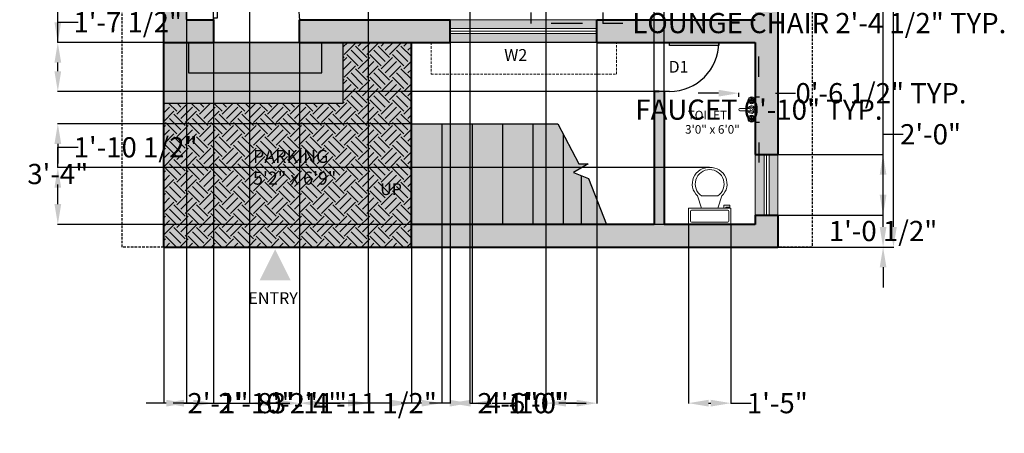
# Model space of a CAD drawing. Units: inches. Extents: x 277 to 728, y 649 to 1132.
# Tile 1 of 4: x 285 to 674, y 649 to 813. Entities that reach past the tile are written whole.
import ezdxf

# ---------------------------------------------------------------- set-up
doc = ezdxf.new("R2010")
doc.units = ezdxf.units.IN
doc.header["$MEASUREMENT"] = 0
doc.linetypes.add('DASHEDX2', pattern=[1.5, 1, -0.5])
for name, color, linetype, lineweight in [('A-ANNO-DIMS', 2, 'Continuous', 18), ('A-ANNO-SYMB', 7, 'Continuous', 18), ('A-ANNO-TEXT', 7, 'Continuous', 18), ('A-AREA-IDEN', 7, 'Continuous', 25), ('A-DOOR', 3, 'Continuous', 25), ('A-FLOR-FIXT', 8, 'Continuous', 18), ('A-FLOR-STRS', 7, 'Continuous', 25), ('A-FLOR-STRS-PATT', 252, 'Continuous', 9), ('A-GLAZ', 4, 'Continuous', 18), ('A-GLAZ-OVHD', 8, 'DASHEDX2', 13), ('A-WALL', 7, 'Continuous', 40), ('A-WALL-PATT', 8, 'Continuous', 13), ('C-PROP', 7, 'DASHEDX2', 25)]:
    doc.layers.add(name, color=color, linetype=linetype, lineweight=lineweight)
for name, color, linetype, lineweight, true_color in [('A-FLOR-FNSH-PATT', 144, 'Continuous', 9, 0x1e788f), ('A-FLOR-PATT', 39, 'Continuous', 9, 0x603913), ('A-GLAZ-PATT', 144, 'Continuous', 13, 0x1e788f)]:
    doc.layers.add(name, color=color, linetype=linetype, lineweight=lineweight, true_color=true_color)
doc.styles.get("Standard").update_dxf_attribs({"font": 'arial.ttf'})
doc.dimstyles.get("Standard").update_dxf_attribs({"dimtxt": 8, "dimasz": 8, "dimexe": 0.18, "dimexo": 0.0625, "dimgap": 0.09, "dimtad": 0, "dimtih": 1, "dimtoh": 1, "dimdec": 0, "dimzin": 0, "dimdsep": 46, "dimlunit": 3, "dimtxsty": 'Standard', "dimcen": 0.09, "dimadec": 0, "dimazin": 0, "dimtfac": 1, "dimtdec": 0, "dimtofl": 0, "dimtmove": 0, "dimatfit": 3, "dimfxl": 1, "dimtolj": 1, "dimtzin": 0, "dimarcsym": 0})

# ---------------------------------------------------------------- blocks, each defined once
blk = doc.blocks.new('*U4')
for p, q in [((0, 0), (0, -6)), ((40, 0), (40, -6))]:
    blk.add_line(p, q)
blk.add_lwpolyline([(0, 0), (0, 40), (1.75, 40), (1.75, 0)], close=True)
blk.add_arc((0, 0), 40, 0, 90)
blk = doc.blocks.new('*U5')
for p, q in [((0, 0), (0, -6)), ((28, 0), (28, -6))]:
    blk.add_line(p, q)
blk.add_lwpolyline([(0, 0), (0, 28), (1.75, 28), (1.75, 0)], close=True)
blk.add_arc((0, 0), 28, 0, 90)
blk = doc.blocks.new('*U16')
for p, q in [((9.5, -6), (9.5, -2)), ((-10, -8.5), (-8, -8.5)), ((-10, -9.5), (-10, -8.5)), ((-7, -9.5), (-10, -9.5)), ((-8, -8.5), (-8, -8)), ((-7, -8), (-7, -9.5)), ((-4, -8), (-6, -14)), ((4, -8), (6, -14)), ((4, -14), (-4, -14))]:
    blk.add_line(p, q)
blk.add_lwpolyline([(10.5, -8), (10.5, 0), (-10.5, 0), (-10.5, -8)], close=True)
for points in [[(-9.5, -2), (-9.5, -6)], [(8.5, -1), (-8.5, -1)], [(-8.5, -7), (8.5, -7)]]:
    blk.add_lwpolyline(points)
for centre, radius, start, end in [((-8.625, -1.875), 0.8839, 81.8699, 188.1301), ((8.625, -1.875), 0.8839, 351.8699, 98.1301), ((-8.625, -6.125), 0.8839, 171.869898, 278.1301), ((8.625, -6.125), 0.8839, 261.8699, 8.1301), ((-0.4772, -19.9188), 8.0953, 133.01722, 273.38), ((0.0374, -19.8731), 7.127, 124.50543, 269.7), ((-0.0373, -19.8731), 7.127, 270.3, 55.4946), ((0.4773, -19.9188), 8.0953, 266.62, 46.9828)]:
    blk.add_arc(centre, radius, start, end)
blk = doc.blocks.new('Faucet - Bathroom top')
for p, q in [((-4.107, 0.125), (-4.375, 0.125)), ((-3.75, 0.4788), (-3.75, 0.75)), ((-3.5, 0.482), (-3.5, 0.75)), ((-3.1461, 0.125), (-2.875, 0.125)), ((3.143, 0.125), (2.875, 0.125)), ((3.5, 0.4788), (3.5, 0.75)), ((3.75, 0.482), (3.75, 0.75)), ((4.1039, 0.125), (4.375, 0.125)), ((-4.1039, -0.125), (-4.375, -0.125)), ((-3.75, -0.4821), (-3.75, -0.75)), ((-3.5, -0.4789), (-3.5, -0.75)), ((-3.143, -0.125), (-2.875, -0.125)), ((-0.5, -0.8639), (-0.5, -4.5)), ((0.5, -4.5), (0.5, -0.8631)), ((3.1461, -0.125), (2.875, -0.125)), ((3.5, -0.4821), (3.5, -0.75)), ((3.75, -0.4789), (3.75, -0.75)), ((4.107, -0.125), (4.375, -0.125))]:
    blk.add_line(p, q)
for centre, radius in [((-3.625, 0), 1.375), ((-4.625, 0), 0.2795), ((-3.625, 0), 0.5), ((-3.625, 1), 0.2795), ((-2.625, 0), 0.2795), ((0, 0), 0.5), ((3.625, 0), 1.375), ((2.625, 0), 0.2795), ((3.625, 0), 0.5), ((3.625, 1), 0.2795), ((4.625, 0), 0.2795), ((-3.625, -1), 0.2795), ((3.625, -1), 0.2795)]:
    blk.add_circle(centre, radius)
for centre, radius, start, end in [((-3.625, 0), 1, 105.2407, 164.2093), ((-3.625, 0), 1, 16.44125, 74.07887), ((0, 0), 1.5, 289.6514, 250.3603), ((0, 0), 1, 300.3431, 239.7554), ((3.625, 0), 1, 106.12, 164.0884), ((3.625, 0), 1, 16.23422, 73.90469), ((-3.625, 0), 1, 196.2342, 253.9047), ((-3.625, 0), 1, 286.12, 344.0884), ((3.625, 0), 1, 196.4413, 254.0789), ((3.625, 0), 1, 285.2407, 344.2093), ((0, -4.5), 0.5, 180, 0)]:
    blk.add_arc(centre, radius, start, end)
blk = doc.blocks.new('Moment Connection - Imperial')
at = {"color": 0}
blk.add_solid([(0, 0.125), (0.125, 0.0625), (0, 0)], dxfattribs=at)
blk = doc.blocks.new('*D21')
at = {"layer": 'A-ANNO-DIMS', "color": 0, "lineweight": -2, "transparency": 16777216}
for p, q in [((598.28, 1083.05), (630.62, 1083.05)), ((630.44, 1075.05), (630.44, 907.23)), ((630.44, 731.05), (630.44, 898.87)), ((598.28, 723.05), (630.62, 723.05))]:
    blk.add_line(p, q, dxfattribs=at)
at = {"layer": 'A-ANNO-DIMS', "color": 0, "transparency": 16777216}
for points in [[(629.11, 1075.05), (631.77, 1075.05), (630.44, 1083.05)], [(629.11, 731.05), (631.77, 731.05), (630.44, 723.05)]]:
    blk.add_solid(points, dxfattribs=at)
at = {"layer": 'Defpoints', "color": 0, "transparency": 16777216}
for p in [(598.22, 1083.05), (598.22, 723.05), (630.44, 723.05)]:
    blk.add_point(p, dxfattribs=at)
at = {"layer": 'A-ANNO-DIMS', "color": 0, "transparency": 16777216, "insert": (630.44, 903.05), "char_height": 8, "attachment_point": 5}
blk.add_mtext("\\A1;30'", dxfattribs=at)
blk = doc.blocks.new('*D27')
at = {"layer": 'A-ANNO-DIMS', "color": 0, "lineweight": -2, "transparency": 16777216}
for p, q in [((577.22, 790.46), (577.22, 798.46)), ((575.78, 782.46), (577.4, 782.46)), ((575.78, 772.46), (577.4, 772.46)), ((577.22, 764.46), (577.22, 756.46))]:
    blk.add_line(p, q, dxfattribs=at)
at = {"layer": 'A-ANNO-DIMS', "color": 0, "transparency": 16777216}
for points in [[(575.89, 790.46), (578.55, 790.46), (577.22, 782.46)], [(575.89, 764.46), (578.55, 764.46), (577.22, 772.46)]]:
    blk.add_solid(points, dxfattribs=at)
at = {"layer": 'Defpoints', "color": 0, "transparency": 16777216}
for p in [(575.72, 782.46), (575.72, 772.46), (577.22, 772.46)]:
    blk.add_point(p, dxfattribs=at)
at = {"layer": 'A-ANNO-DIMS', "color": 0, "transparency": 16777216, "insert": (577.22, 777.46), "char_height": 8, "attachment_point": 5}
blk.add_mtext('\\A1;FAUCET 0\'-10" TYP.', dxfattribs=at)
blk = doc.blocks.new('*D28')
at = {"layer": 'A-ANNO-DIMS', "color": 0, "lineweight": -2, "transparency": 16777216}
for p, q in [((561.22, 783.96), (553.22, 783.96)), ((569.22, 782.52), (569.22, 784.14)), ((575.72, 782.52), (575.72, 784.14)), ((583.72, 783.96), (591.72, 783.96))]:
    blk.add_line(p, q, dxfattribs=at)
at = {"layer": 'A-ANNO-DIMS', "color": 0, "transparency": 16777216}
for points in [[(561.22, 785.29), (561.22, 782.62), (569.22, 783.96)], [(583.72, 785.29), (583.72, 782.62), (575.72, 783.96)]]:
    blk.add_solid(points, dxfattribs=at)
at = {"layer": 'Defpoints', "color": 0, "transparency": 16777216}
for p in [(575.72, 783.96), (569.22, 782.46), (575.72, 782.46)]:
    blk.add_point(p, dxfattribs=at)
at = {"layer": 'A-ANNO-DIMS', "color": 0, "transparency": 16777216, "insert": (625.51, 783.96), "char_height": 8, "attachment_point": 5}
blk.add_mtext('\\A1;0\'-6 1/2" TYP.', dxfattribs=at)
blk = doc.blocks.new('*D29')
at = {"layer": 'A-ANNO-DIMS', "color": 0, "lineweight": -2, "transparency": 16777216}
for p, q in [((486.97, 815.91), (486.97, 811.53)), ((515.41, 815.91), (515.41, 811.53)), ((494.97, 811.71), (507.41, 811.71)), ((515.41, 811.71), (523.41, 811.71))]:
    blk.add_line(p, q, dxfattribs=at)
at = {"layer": 'A-ANNO-DIMS', "color": 0, "transparency": 16777216}
for points in [[(494.97, 813.04), (494.97, 810.37), (486.97, 811.71)], [(507.41, 813.04), (507.41, 810.37), (515.41, 811.71)]]:
    blk.add_solid(points, dxfattribs=at)
at = {"layer": 'Defpoints', "color": 0, "transparency": 16777216}
for p in [(486.97, 815.97), (515.41, 815.97), (515.41, 811.71)]:
    blk.add_point(p, dxfattribs=at)
at = {"layer": 'A-ANNO-DIMS', "color": 0, "transparency": 16777216, "insert": (601.11, 811.71), "char_height": 8, "attachment_point": 5}
blk.add_mtext('\\A1;LOUNGE CHAIR 2\'-4 1/2" TYP.', dxfattribs=at)
blk = doc.blocks.new('*D48')
at = {"layer": 'A-ANNO-DIMS', "color": 0, "lineweight": -2, "transparency": 16777216}
for p, q in [((584.78, 1071.05), (626.51, 1071.05)), ((626.33, 1063.05), (626.33, 901.23)), ((626.33, 731.05), (626.33, 892.88)), ((584.78, 723.05), (626.51, 723.05))]:
    blk.add_line(p, q, dxfattribs=at)
at = {"layer": 'A-ANNO-DIMS', "color": 0, "transparency": 16777216}
for points in [[(625, 1063.05), (627.67, 1063.05), (626.33, 1071.05)], [(625, 731.05), (627.67, 731.05), (626.33, 723.05)]]:
    blk.add_solid(points, dxfattribs=at)
at = {"layer": 'Defpoints', "color": 0, "transparency": 16777216}
for p in [(584.72, 1071.05), (626.33, 1071.05), (584.72, 723.05)]:
    blk.add_point(p, dxfattribs=at)
at = {"layer": 'A-ANNO-DIMS', "color": 0, "transparency": 16777216, "insert": (626.33, 897.05), "char_height": 8, "attachment_point": 5}
blk.add_mtext('\\A1;29\'-0"', dxfattribs=at)
blk = doc.blocks.new('*D52')
at = {"layer": 'A-ANNO-DIMS', "color": 0, "lineweight": -2, "transparency": 16777216}
for p, q in [((341.66, 942.05), (299.63, 942.05)), ((299.81, 934.05), (299.81, 877.23)), ((299.81, 812.05), (299.81, 868.88)), ((341.66, 804.05), (299.63, 804.05))]:
    blk.add_line(p, q, dxfattribs=at)
at = {"layer": 'A-ANNO-DIMS', "color": 0, "transparency": 16777216}
for points in [[(298.48, 934.05), (301.15, 934.05), (299.81, 942.05)], [(298.48, 812.05), (301.15, 812.05), (299.81, 804.05)]]:
    blk.add_solid(points, dxfattribs=at)
at = {"layer": 'Defpoints', "color": 0, "transparency": 16777216}
for p in [(299.81, 942.05), (341.72, 942.05), (341.72, 804.05)]:
    blk.add_point(p, dxfattribs=at)
at = {"layer": 'A-ANNO-DIMS', "color": 0, "transparency": 16777216, "insert": (299.81, 873.05), "char_height": 8, "attachment_point": 5}
blk.add_mtext('\\A1;11\'-6"', dxfattribs=at)
blk = doc.blocks.new('*D55')
at = {"layer": 'A-ANNO-DIMS', "color": 0, "lineweight": -2, "transparency": 16777216}
for p, q in [((626.33, 759.7), (626.33, 767.7)), ((626.33, 767.7), (634.33, 767.7)), ((584.78, 759.7), (626.51, 759.7)), ((626.33, 743.74), (626.33, 751.7)), ((584.78, 735.74), (626.51, 735.74))]:
    blk.add_line(p, q, dxfattribs=at)
at = {"layer": 'A-ANNO-DIMS', "color": 0, "transparency": 16777216}
for points in [[(625, 751.7), (627.67, 751.7), (626.33, 759.7)], [(625, 743.74), (627.67, 743.74), (626.33, 735.74)]]:
    blk.add_solid(points, dxfattribs=at)
at = {"layer": 'Defpoints', "color": 0, "transparency": 16777216}
for p in [(584.72, 759.7), (626.33, 759.7), (584.72, 735.74)]:
    blk.add_point(p, dxfattribs=at)
at = {"layer": 'A-ANNO-DIMS', "color": 0, "transparency": 16777216, "insert": (645.12, 767.7), "char_height": 8, "attachment_point": 5}
blk.add_mtext('\\A1;2\'-0"', dxfattribs=at)
blk = doc.blocks.new('*D56')
at = {"layer": 'A-ANNO-DIMS', "color": 0, "lineweight": -2, "transparency": 16777216}
for p, q in [((626.33, 743.74), (626.33, 751.74)), ((584.78, 735.74), (626.51, 735.74)), ((584.78, 723.05), (626.51, 723.05)), ((626.33, 715.05), (626.33, 707.05))]:
    blk.add_line(p, q, dxfattribs=at)
at = {"layer": 'A-ANNO-DIMS', "color": 0, "transparency": 16777216}
for points in [[(625, 743.74), (627.67, 743.74), (626.33, 735.74)], [(625, 715.05), (627.67, 715.05), (626.33, 723.05)]]:
    blk.add_solid(points, dxfattribs=at)
at = {"layer": 'Defpoints', "color": 0, "transparency": 16777216}
for p in [(584.72, 735.74), (626.33, 735.74), (584.72, 723.05)]:
    blk.add_point(p, dxfattribs=at)
at = {"layer": 'A-ANNO-DIMS', "color": 0, "transparency": 16777216, "insert": (626.33, 729.4), "char_height": 8, "attachment_point": 5}
blk.add_mtext('\\A1;1\'-0 1/2"', dxfattribs=at)
blk = doc.blocks.new('*D57')
at = {"layer": 'A-ANNO-DIMS', "color": 0, "lineweight": -2, "transparency": 16777216}
for p, q in [((341.72, 722.99), (341.72, 661.09)), ((439.72, 722.99), (439.72, 661.09)), ((349.72, 661.27), (379.99, 661.27)), ((431.72, 661.27), (401.45, 661.27))]:
    blk.add_line(p, q, dxfattribs=at)
at = {"layer": 'A-ANNO-DIMS', "color": 0, "transparency": 16777216}
for points in [[(349.72, 662.6), (349.72, 659.93), (341.72, 661.27)], [(431.72, 662.6), (431.72, 659.93), (439.72, 661.27)]]:
    blk.add_solid(points, dxfattribs=at)
at = {"layer": 'Defpoints', "color": 0, "transparency": 16777216}
for p in [(341.72, 723.05), (439.72, 723.05), (439.72, 661.27)]:
    blk.add_point(p, dxfattribs=at)
at = {"layer": 'A-ANNO-DIMS', "color": 0, "transparency": 16777216, "insert": (390.72, 661.27), "char_height": 8, "attachment_point": 5}
blk.add_mtext('\\A1;8\'-2"', dxfattribs=at)
blk = doc.blocks.new('*D58')
at = {"layer": 'A-ANNO-DIMS', "color": 0, "lineweight": -2, "transparency": 16777216}
for p, q in [((342.72, 1117.04), (334.72, 1117.04)), ((350.72, 813.11), (350.72, 1117.22)), ((361.43, 813.11), (361.43, 1117.22)), ((369.43, 1117.04), (377.43, 1117.04))]:
    blk.add_line(p, q, dxfattribs=at)
at = {"layer": 'A-ANNO-DIMS', "color": 0, "transparency": 16777216}
for points in [[(342.72, 1118.37), (342.72, 1115.71), (350.72, 1117.04)], [(369.43, 1118.37), (369.43, 1115.71), (361.43, 1117.04)]]:
    blk.add_solid(points, dxfattribs=at)
at = {"layer": 'Defpoints', "color": 0, "transparency": 16777216}
for p in [(361.43, 1117.04), (350.72, 813.05), (361.43, 813.05)]:
    blk.add_point(p, dxfattribs=at)
at = {"layer": 'A-ANNO-DIMS', "color": 0, "transparency": 16777216, "insert": (400.59, 1117.04), "char_height": 8, "attachment_point": 5}
blk.add_mtext('\\A1;0\'-10 1/2"', dxfattribs=at)
blk = doc.blocks.new('*D59')
at = {"layer": 'A-ANNO-DIMS', "color": 0, "lineweight": -2, "transparency": 16777216}
for p, q in [((361.43, 803.99), (361.43, 661.09)), ((395.5, 803.99), (395.5, 661.09)), ((353.43, 661.27), (345.43, 661.27)), ((403.5, 661.27), (411.5, 661.27))]:
    blk.add_line(p, q, dxfattribs=at)
at = {"layer": 'A-ANNO-DIMS', "color": 0, "transparency": 16777216}
for points in [[(353.43, 662.6), (353.43, 659.93), (361.43, 661.27)], [(403.5, 662.6), (403.5, 659.93), (395.5, 661.27)]]:
    blk.add_solid(points, dxfattribs=at)
at = {"layer": 'Defpoints', "color": 0, "transparency": 16777216}
for p in [(361.43, 804.05), (395.5, 804.05), (395.5, 661.27)]:
    blk.add_point(p, dxfattribs=at)
at = {"layer": 'A-ANNO-DIMS', "color": 0, "transparency": 16777216, "insert": (378.46, 661.27), "char_height": 8, "attachment_point": 5}
blk.add_mtext('\\A1;2\'-10"', dxfattribs=at)
blk = doc.blocks.new('*D60')
at = {"layer": 'A-ANNO-DIMS', "color": 0, "lineweight": -2, "transparency": 16777216}
for p, q in [((395.5, 803.99), (395.5, 661.09)), ((455.1, 803.99), (455.1, 661.09)), ((387.5, 661.27), (379.5, 661.27)), ((463.1, 661.27), (471.1, 661.27))]:
    blk.add_line(p, q, dxfattribs=at)
at = {"layer": 'A-ANNO-DIMS', "color": 0, "transparency": 16777216}
for points in [[(387.5, 662.6), (387.5, 659.93), (395.5, 661.27)], [(463.1, 662.6), (463.1, 659.93), (455.1, 661.27)]]:
    blk.add_solid(points, dxfattribs=at)
at = {"layer": 'Defpoints', "color": 0, "transparency": 16777216}
for p in [(395.5, 804.05), (455.1, 804.05), (455.1, 661.27)]:
    blk.add_point(p, dxfattribs=at)
at = {"layer": 'A-ANNO-DIMS', "color": 0, "transparency": 16777216, "insert": (425.3, 661.27), "char_height": 8, "attachment_point": 5}
blk.add_mtext('\\A1;4\'-11 1/2"', dxfattribs=at)
blk = doc.blocks.new('*D61')
at = {"layer": 'A-ANNO-DIMS', "color": 0, "lineweight": -2, "transparency": 16777216}
for p, q in [((455.1, 803.99), (455.1, 661.09)), ((513.09, 803.99), (513.09, 661.09)), ((463.1, 661.27), (470.11, 661.27)), ((505.09, 661.27), (498.09, 661.27))]:
    blk.add_line(p, q, dxfattribs=at)
at = {"layer": 'A-ANNO-DIMS', "color": 0, "transparency": 16777216}
for points in [[(463.1, 662.6), (463.1, 659.93), (455.1, 661.27)], [(505.09, 662.6), (505.09, 659.93), (513.09, 661.27)]]:
    blk.add_solid(points, dxfattribs=at)
at = {"layer": 'Defpoints', "color": 0, "transparency": 16777216}
for p in [(455.1, 804.05), (513.09, 804.05), (513.09, 661.27)]:
    blk.add_point(p, dxfattribs=at)
at = {"layer": 'A-ANNO-DIMS', "color": 0, "transparency": 16777216, "insert": (484.1, 661.27), "char_height": 8, "attachment_point": 5}
blk.add_mtext('\\A1;4\'-10"', dxfattribs=at)
blk = doc.blocks.new('*D62')
at = {"layer": 'A-ANNO-DIMS', "color": 0, "lineweight": -2, "transparency": 16777216}
for p, q in [((462.81, 941.99), (462.81, 661.09)), ((492.89, 941.99), (492.89, 661.09)), ((454.81, 661.27), (446.81, 661.27)), ((500.89, 661.27), (508.89, 661.27))]:
    blk.add_line(p, q, dxfattribs=at)
at = {"layer": 'A-ANNO-DIMS', "color": 0, "transparency": 16777216}
for points in [[(454.81, 662.6), (454.81, 659.93), (462.81, 661.27)], [(500.89, 662.6), (500.89, 659.93), (492.89, 661.27)]]:
    blk.add_solid(points, dxfattribs=at)
at = {"layer": 'Defpoints', "color": 0, "transparency": 16777216}
for p in [(462.81, 942.05), (492.89, 942.05), (492.89, 661.27)]:
    blk.add_point(p, dxfattribs=at)
at = {"layer": 'A-ANNO-DIMS', "color": 0, "transparency": 16777216, "insert": (477.85, 661.27), "char_height": 8, "attachment_point": 5}
blk.add_mtext('\\A1;2\'-6"', dxfattribs=at)
blk = doc.blocks.new('*D63')
at = {"layer": 'A-ANNO-DIMS', "color": 0, "lineweight": -2, "transparency": 16777216}
for p, q in [((375.63, 932.99), (375.63, 661.09)), ((422.67, 932.99), (422.67, 661.09)), ((383.63, 661.27), (385.32, 661.27)), ((414.67, 661.27), (412.98, 661.27))]:
    blk.add_line(p, q, dxfattribs=at)
at = {"layer": 'A-ANNO-DIMS', "color": 0, "transparency": 16777216}
for points in [[(383.63, 662.6), (383.63, 659.93), (375.63, 661.27)], [(414.67, 662.6), (414.67, 659.93), (422.67, 661.27)]]:
    blk.add_solid(points, dxfattribs=at)
at = {"layer": 'Defpoints', "color": 0, "transparency": 16777216}
for p in [(375.63, 933.05), (422.67, 933.05), (422.67, 661.27)]:
    blk.add_point(p, dxfattribs=at)
at = {"layer": 'A-ANNO-DIMS', "color": 0, "transparency": 16777216, "insert": (399.15, 661.27), "char_height": 8, "attachment_point": 5}
blk.add_mtext('\\A1;3\'-11"', dxfattribs=at)
blk = doc.blocks.new('*D64')
at = {"layer": 'A-ANNO-DIMS', "color": 0, "lineweight": -2, "transparency": 16777216}
for p, q in [((299.81, 804.05), (299.81, 812.05)), ((299.81, 812.05), (307.81, 812.05)), ((540.6, 804.05), (299.63, 804.05)), ((299.81, 792.62), (299.81, 796.05)), ((535.66, 784.62), (299.63, 784.62))]:
    blk.add_line(p, q, dxfattribs=at)
at = {"layer": 'A-ANNO-DIMS', "color": 0, "transparency": 16777216}
for points in [[(298.48, 796.05), (301.15, 796.05), (299.81, 804.05)], [(298.48, 792.62), (301.15, 792.62), (299.81, 784.62)]]:
    blk.add_solid(points, dxfattribs=at)
at = {"layer": 'Defpoints', "color": 0, "transparency": 16777216}
for p in [(299.81, 804.05), (540.67, 804.05), (535.72, 784.62)]:
    blk.add_point(p, dxfattribs=at)
at = {"layer": 'A-ANNO-DIMS', "color": 0, "transparency": 16777216, "insert": (327.48, 812.05), "char_height": 8, "attachment_point": 5}
blk.add_mtext('\\A1;1\'-7 1/2"', dxfattribs=at)
blk = doc.blocks.new('*D66')
at = {"layer": 'A-ANNO-DIMS', "color": 0, "lineweight": -2, "transparency": 16777216}
for p, q in [((350.72, 932.99), (350.72, 661.09)), ((375.63, 932.99), (375.63, 661.09)), ((342.72, 661.27), (334.72, 661.27)), ((383.63, 661.27), (391.63, 661.27))]:
    blk.add_line(p, q, dxfattribs=at)
at = {"layer": 'A-ANNO-DIMS', "color": 0, "transparency": 16777216}
for points in [[(342.72, 662.6), (342.72, 659.93), (350.72, 661.27)], [(383.63, 662.6), (383.63, 659.93), (375.63, 661.27)]]:
    blk.add_solid(points, dxfattribs=at)
at = {"layer": 'Defpoints', "color": 0, "transparency": 16777216}
for p in [(350.72, 933.05), (375.63, 933.05), (375.63, 661.27)]:
    blk.add_point(p, dxfattribs=at)
at = {"layer": 'A-ANNO-DIMS', "color": 0, "transparency": 16777216, "insert": (363.17, 661.27), "char_height": 8, "attachment_point": 5}
blk.add_mtext('\\A1;2\'-1"', dxfattribs=at)
blk = doc.blocks.new('*D69')
at = {"layer": 'A-ANNO-DIMS', "color": 0, "lineweight": -2, "transparency": 16777216}
for p, q in [((451.72, 731.99), (451.72, 661.09)), ((463.72, 731.99), (463.72, 661.09)), ((443.72, 661.27), (435.72, 661.27)), ((471.72, 661.27), (479.72, 661.27))]:
    blk.add_line(p, q, dxfattribs=at)
at = {"layer": 'A-ANNO-DIMS', "color": 0, "transparency": 16777216}
for points in [[(443.72, 662.6), (443.72, 659.93), (451.72, 661.27)], [(471.72, 662.6), (471.72, 659.93), (463.72, 661.27)]]:
    blk.add_solid(points, dxfattribs=at)
at = {"layer": 'Defpoints', "color": 0, "transparency": 16777216}
for p in [(451.72, 732.05), (463.72, 732.05), (463.72, 661.27)]:
    blk.add_point(p, dxfattribs=at)
at = {"layer": 'A-ANNO-DIMS', "color": 0, "transparency": 16777216, "insert": (490.06, 661.27), "char_height": 8, "attachment_point": 5}
blk.add_mtext('\\A1;1\'-0"', dxfattribs=at)
blk = doc.blocks.new('*D70')
at = {"layer": 'A-ANNO-DIMS', "color": 0, "lineweight": -2, "transparency": 16777216}
for p, q in [((439.66, 771.89), (299.63, 771.89)), ((299.81, 763.89), (299.81, 756.15)), ((299.81, 740.05), (299.81, 747.79)), ((439.66, 732.05), (299.63, 732.05))]:
    blk.add_line(p, q, dxfattribs=at)
at = {"layer": 'A-ANNO-DIMS', "color": 0, "transparency": 16777216}
for points in [[(298.48, 763.89), (301.15, 763.89), (299.81, 771.89)], [(298.48, 740.05), (301.15, 740.05), (299.81, 732.05)]]:
    blk.add_solid(points, dxfattribs=at)
at = {"layer": 'Defpoints', "color": 0, "transparency": 16777216}
for p in [(299.81, 771.89), (439.72, 771.89), (439.72, 732.05)]:
    blk.add_point(p, dxfattribs=at)
at = {"layer": 'A-ANNO-DIMS', "color": 0, "transparency": 16777216, "insert": (299.81, 751.97), "char_height": 8, "attachment_point": 5}
blk.add_mtext('\\A1;3\'-4"', dxfattribs=at)
blk = doc.blocks.new('*D71')
at = {"layer": 'A-ANNO-DIMS', "color": 0, "lineweight": -2, "transparency": 16777216}
for p, q in [((549.29, 731.99), (549.29, 661.09)), ((566.15, 731.99), (566.15, 661.09)), ((557.29, 661.27), (558.15, 661.27)), ((566.15, 661.27), (574.15, 661.27))]:
    blk.add_line(p, q, dxfattribs=at)
at = {"layer": 'A-ANNO-DIMS', "color": 0, "transparency": 16777216}
for points in [[(557.29, 662.6), (557.29, 659.93), (549.29, 661.27)], [(558.15, 662.6), (558.15, 659.93), (566.15, 661.27)]]:
    blk.add_solid(points, dxfattribs=at)
at = {"layer": 'Defpoints', "color": 0, "transparency": 16777216}
for p in [(549.29, 732.05), (566.15, 732.05), (566.15, 661.27)]:
    blk.add_point(p, dxfattribs=at)
at = {"layer": 'A-ANNO-DIMS', "color": 0, "transparency": 16777216, "insert": (584.5, 661.27), "char_height": 8, "attachment_point": 5}
blk.add_mtext('\\A1;1\'-5"', dxfattribs=at)
blk = doc.blocks.new('*D72')
at = {"layer": 'A-ANNO-DIMS', "color": 0, "lineweight": -2, "transparency": 16777216}
for p, q in [((299.81, 754.54), (299.81, 762.54)), ((299.81, 762.54), (307.81, 762.54)), ((557.66, 754.54), (299.63, 754.54)), ((299.81, 740.05), (299.81, 746.54)), ((549.22, 732.05), (299.63, 732.05))]:
    blk.add_line(p, q, dxfattribs=at)
at = {"layer": 'A-ANNO-DIMS', "color": 0, "transparency": 16777216}
for points in [[(298.48, 746.54), (301.15, 746.54), (299.81, 754.54)], [(298.48, 740.05), (301.15, 740.05), (299.81, 732.05)]]:
    blk.add_solid(points, dxfattribs=at)
at = {"layer": 'Defpoints', "color": 0, "transparency": 16777216}
for p in [(299.81, 754.54), (557.72, 754.54), (549.29, 732.05)]:
    blk.add_point(p, dxfattribs=at)
at = {"layer": 'A-ANNO-DIMS', "color": 0, "transparency": 16777216, "insert": (330.59, 762.54), "char_height": 8, "attachment_point": 5}
blk.add_mtext('\\A1;1\'-10 1/2"', dxfattribs=at)
blk = doc.blocks.new('*D75')
at = {"layer": 'A-ANNO-DIMS', "color": 0, "lineweight": -2, "transparency": 16777216}
for p, q in [((527.72, 1117.04), (519.72, 1117.04)), ((535.72, 784.69), (535.72, 1117.22)), ((539.72, 784.69), (539.72, 1117.22)), ((547.72, 1117.04), (555.72, 1117.04))]:
    blk.add_line(p, q, dxfattribs=at)
at = {"layer": 'A-ANNO-DIMS', "color": 0, "transparency": 16777216}
for points in [[(527.72, 1118.37), (527.72, 1115.71), (535.72, 1117.04)], [(547.72, 1118.37), (547.72, 1115.71), (539.72, 1117.04)]]:
    blk.add_solid(points, dxfattribs=at)
at = {"layer": 'Defpoints', "color": 0, "transparency": 16777216}
for p in [(535.72, 1117.04), (535.72, 784.62), (539.72, 784.62)]:
    blk.add_point(p, dxfattribs=at)
at = {"layer": 'A-ANNO-DIMS', "color": 0, "transparency": 16777216, "insert": (509, 1117.04), "char_height": 8, "attachment_point": 5}
blk.add_mtext('\\A1;0\'-4"', dxfattribs=at)

msp = doc.modelspace()

# ---------------------------------------------------------------- hatches: boundary and pattern name
at = {"layer": 'A-FLOR-FNSH-PATT'}
h = msp.add_hatch(color=256, dxfattribs=at)
h.dxf.hatch_style = 1
h.paths.add_polyline_path([(439.72, 723.05), (439.72, 804.05), (412.73, 804.05), (412.73, 780.05), (341.72, 780.05), (341.72, 723.05)])
h.paths.add_polyline_path([(425.67, 741.1), (437.05, 741.1), (437.05, 750.7), (425.67, 750.7)], flags=24)
h.paths.add_polyline_path([(375.21, 744.82), (410.28, 744.82), (410.28, 764.1), (375.21, 764.1)], flags=24)
at = {"layer": 'A-FLOR-PATT'}
h = msp.add_hatch(dxfattribs=at)
h.set_pattern_fill('EARTH', color=256, angle=45)
h.set_pattern_definition([(45, (0, 0), (0, 8.980256), [6.35, -6.35]), (45, (-1.684, 1.684), (0, 8.980256), [6.35, -6.35]), (45, (-3.3676, 3.3676), (0, 8.980256), [6.35, -6.35]), (135, (-3.3676, 4.49), (-8.980256, 0), [6.35, -6.35]), (135, (-1.684, 6.174), (-8.980256, 0), [6.35, -6.35]), (135, (0, 7.858), (-8.980256, 0), [6.35, -6.35])])
h.paths.add_polyline_path([(439.72, 723.05), (439.72, 804.05), (412.73, 804.05), (412.73, 780.05), (341.72, 780.05), (341.72, 723.05)])
h.paths.add_polyline_path([(425.67, 741.1), (437.05, 741.1), (437.05, 750.7), (425.67, 750.7)], flags=24)
h.paths.add_polyline_path([(375.21, 744.82), (410.28, 744.82), (410.28, 764.1), (375.21, 764.1)], flags=24)
at = {"layer": 'A-FLOR-STRS-PATT'}
h = msp.add_hatch(color=256, dxfattribs=at)
h.dxf.hatch_style = 1
h.paths.add_polyline_path([(351.58, 792.05), (351.58, 804.05), (341.72, 804.05), (341.72, 780.05), (412.73, 780.05), (412.73, 804.05), (404.3, 804.05), (404.3, 792.05)])
h = msp.add_hatch(color=256, dxfattribs=at)
h.dxf.hatch_style = 1
h.paths.add_polyline_path([(404.3, 792.05), (404.3, 804.05), (395.5, 804.05), (361.43, 804.05), (351.58, 804.05), (351.58, 792.05)])
h = msp.add_hatch(color=256, dxfattribs=at)
h.dxf.hatch_style = 1
h.paths.add_polyline_path([(451.72, 771.89), (439.72, 771.89), (439.72, 732.05), (451.72, 732.05)])
h = msp.add_hatch(color=256, dxfattribs=at)
h.dxf.hatch_style = 1
h.paths.add_polyline_path([(451.72, 732.05), (463.72, 732.05), (463.72, 771.89), (451.72, 771.89)])
h = msp.add_hatch(color=256, dxfattribs=at)
h.dxf.hatch_style = 1
h.paths.add_polyline_path([(475.72, 771.89), (463.72, 771.89), (463.72, 732.05), (475.72, 732.05)])
h = msp.add_hatch(color=256, dxfattribs=at)
h.dxf.hatch_style = 1
h.paths.add_polyline_path([(475.72, 732.05), (487.72, 732.05), (487.72, 771.89), (475.72, 771.89)])
h = msp.add_hatch(color=256, dxfattribs=at)
h.dxf.hatch_style = 1
h.paths.add_polyline_path([(499.72, 767.86), (497.59, 771.89), (487.72, 771.89), (487.72, 732.05), (499.72, 732.05)])
h = msp.add_hatch(color=256, dxfattribs=at)
h.dxf.hatch_style = 1
h.paths.add_polyline_path([(499.72, 732.05), (506.83, 732.05), (506.83, 751.34), (503.84, 752.51), (509.6, 755.97), (506, 755.97), (499.72, 767.86)])
h = msp.add_hatch(color=256, dxfattribs=at)
h.dxf.hatch_style = 1
h.paths.add_polyline_path([(506.83, 732.05), (516.92, 732.05), (509.79, 750.18), (506.83, 751.34)])
at = {"layer": 'A-GLAZ-PATT'}
h = msp.add_hatch(color=256, dxfattribs=at)
h.dxf.hatch_style = 1
h.paths.add_polyline_path([(513.09, 809.55), (513.09, 813.05), (455.1, 813.05), (455.1, 809.55)])
h = msp.add_hatch(color=256, dxfattribs=at)
h.dxf.hatch_style = 1
h.paths.add_polyline_path([(513.09, 804.05), (513.09, 807.55), (455.1, 807.55), (455.1, 804.05)])
h = msp.add_hatch(color=256, dxfattribs=at)
h.dxf.hatch_style = 1
h.paths.add_polyline_path([(579.22, 759.7), (575.72, 759.7), (575.72, 735.74), (579.22, 735.74)])
h = msp.add_hatch(color=256, dxfattribs=at)
h.dxf.hatch_style = 1
h.paths.add_polyline_path([(581.22, 735.74), (584.72, 735.74), (584.72, 759.7), (581.22, 759.7)])
at = {"layer": 'A-WALL-PATT'}
h = msp.add_hatch(color=256, dxfattribs=at)
h.dxf.hatch_style = 1
h.paths.add_polyline_path([(361.43, 804.05), (361.43, 813.05), (350.72, 813.05), (350.72, 933.05), (375.63, 933.05), (375.63, 942.05), (350.72, 942.05), (341.72, 942.05), (341.72, 804.05)])
h = msp.add_hatch(color=256, dxfattribs=at)
h.dxf.hatch_style = 1
h.paths.add_polyline_path([(513.09, 813.05), (513.09, 804.05), (575.72, 804.05), (575.72, 759.7), (584.72, 759.7), (584.72, 848.91), (575.72, 848.91), (575.72, 813.05)])
h = msp.add_hatch(color=256, dxfattribs=at)
h.dxf.hatch_style = 1
h.paths.add_polyline_path([(395.5, 813.05), (395.5, 804.05), (455.1, 804.05), (455.1, 813.05)])
h = msp.add_hatch(color=256, dxfattribs=at)
h.dxf.hatch_style = 1
h.paths.add_polyline_path([(584.72, 723.05), (584.72, 735.74), (575.72, 735.74), (575.72, 732.05), (539.72, 732.05), (539.72, 784.62), (537.72, 784.62), (535.72, 784.62), (535.72, 732.05), (439.72, 732.05), (439.72, 723.05)])

# ---------------------------------------------------------------- linework, layer by layer
at = {"layer": 'A-DOOR'}
msp.add_line((361.43, 804.05), (395.5, 804.05), dxfattribs=at)
at = {"layer": 'A-FLOR-STRS'}
for p, q in [((341.72, 804.05), (341.72, 780.05)), ((351.58, 804.05), (351.58, 792.05)), ((404.3, 792.05), (404.3, 804.05)), ((412.73, 780.05), (412.73, 804.05)), ((351.58, 792.05), (404.3, 792.05)), ((341.72, 780.05), (412.73, 780.05)), ((439.72, 771.89), (497.59, 771.89)), ((439.72, 771.89), (451.72, 771.89)), ((451.72, 771.89), (451.72, 732.05)), ((463.72, 771.89), (463.72, 732.05)), ((475.72, 771.89), (475.72, 732.05)), ((487.72, 771.89), (487.72, 732.05)), ((497.59, 771.89), (506, 755.97)), ((499.72, 767.86), (499.72, 732.05)), ((509.6, 755.97), (503.84, 752.51)), ((506, 755.97), (509.6, 755.97)), ((503.84, 752.51), (509.79, 750.18)), ((506.83, 751.34), (506.83, 732.05)), ((509.79, 750.18), (516.92, 732.05))]:
    msp.add_line(p, q, dxfattribs=at)
at = {"layer": 'A-GLAZ'}
for p, q in [((455.1, 813.05), (513.09, 813.05)), ((455.1, 809.55), (513.09, 809.55)), ((455.1, 808.55), (513.09, 808.55)), ((455.1, 807.55), (513.09, 807.55)), ((455.1, 804.05), (513.09, 804.05)), ((575.72, 759.7), (575.72, 735.74)), ((579.22, 759.7), (579.22, 735.74)), ((580.22, 759.7), (580.22, 735.74)), ((581.22, 759.7), (581.22, 735.74)), ((584.72, 759.7), (584.72, 735.74))]:
    msp.add_line(p, q, dxfattribs=at)
at = {"layer": 'A-GLAZ-OVHD'}
for p, q in [((447.51, 804.05), (447.51, 791.49)), ((520.9, 791.49), (520.9, 804.05)), ((447.51, 791.49), (520.9, 791.49))]:
    msp.add_line(p, q, dxfattribs=at)
at = {"layer": 'A-WALL'}
for p, q in [((341.72, 723.05), (341.72, 942.05)), ((584.72, 848.91), (584.72, 759.7)), ((350.72, 813.05), (361.43, 813.05)), ((361.43, 813.05), (361.43, 804.05)), ((395.5, 804.05), (395.5, 813.05)), ((395.5, 813.05), (455.1, 813.05)), ((455.1, 804.05), (455.1, 813.05)), ((513.09, 804.05), (513.09, 813.05)), ((513.09, 813.05), (575.72, 813.05)), ((341.72, 804.05), (361.43, 804.05)), ((395.5, 804.05), (455.1, 804.05)), ((439.72, 723.05), (439.72, 804.05)), ((513.09, 804.05), (575.72, 804.05)), ((575.72, 804.05), (575.72, 759.7)), ((535.72, 784.62), (535.72, 732.05)), ((537.72, 784.62), (535.72, 784.62)), ((539.72, 784.62), (539.72, 732.05)), ((575.72, 759.7), (584.72, 759.7)), ((575.72, 735.74), (584.72, 735.74)), ((575.72, 735.74), (575.72, 732.05)), ((584.72, 735.74), (584.72, 723.05)), ((535.72, 732.05), (439.72, 732.05)), ((575.72, 732.05), (539.72, 732.05)), ((341.72, 723.05), (584.72, 723.05))]:
    msp.add_line(p, q, dxfattribs=at)
at = {"layer": 'C-PROP'}
for p, q in [((325.22, 723.05), (325.22, 1083.05)), ((598.22, 1083.05), (598.22, 723.05)), ((598.22, 723.05), (325.22, 723.05)), ((584.72, 723.05), (325.22, 723.05))]:
    msp.add_line(p, q, dxfattribs=at)

# ---------------------------------------------------------------- block references
at = {"layer": 'A-ANNO-SYMB', "xscale": 98.23354267377717, "yscale": 98.23354267377717, "zscale": 98.23354267377717, "rotation": 90}
msp.add_blockref('Moment Connection - Imperial', (391.93, 709.89), dxfattribs=at)
at = {"layer": 'A-DOOR', "xscale": 0.8508858402266032, "yscale": 0.8508858402266032, "zscale": 0.8508858402266032}
msp.add_blockref('*U4', (361.43, 813.66), dxfattribs=at)
at = {"layer": 'A-DOOR', "xscale": 0.6938229261938118, "yscale": 0.6938229261938118, "zscale": 0.6938229261938118, "rotation": 270}
msp.add_blockref('*U5', (541.88, 804.05), dxfattribs=at)
at = {"layer": 'A-FLOR-FIXT', "rotation": 270}
msp.add_blockref('Faucet - Bathroom top', (574.22, 777.46), dxfattribs=at)
at = {"layer": 'A-FLOR-FIXT', "xscale": 0.8030771595476377, "yscale": 0.8030771595476377, "zscale": 0.8030771595476377, "rotation": 180}
msp.add_blockref('*U16', (557.72, 732.05), dxfattribs=at)

# ---------------------------------------------------------------- texts
at = {"layer": 'A-ANNO-TEXT', "char_height": 4.66, "attachment_point": 1}
for s, insert in [('W2', (476.44, 801.42)), ('D1', (541.46, 796.74)), ('UP', (427.35, 748.3)), ('ENTRY', (375.21, 705.18))]:
    msp.add_mtext_dynamic_manual_height_columns(s, width=6.3557, gutter_width=23.3, heights=[0], dxfattribs=dict(at, insert=insert))
at = {"layer": 'A-AREA-IDEN', "attachment_point": 1}
for s, width, gutter_width, heights, insert, char_height in [(' TOILET\\P3\'0" x 6\'0"', 41.8272, 16.99, [9.2], (547.98, 776.99), 3.3979), ('PARKING\\P5\'2" x 6\'9"', 63.6015, 25.83, [0], (377.06, 761.53), 5.1668)]:
    msp.add_mtext_dynamic_manual_height_columns(s, width=width, gutter_width=gutter_width, heights=heights, dxfattribs=dict(at, insert=insert, char_height=char_height))

# ---------------------------------------------------------------- dimensions: what is measured, and where the dimension line sits
at = {"layer": 'A-ANNO-DIMS'}
for base, p1, p2, picture, middle in [((361.43, 1117.04), (350.72, 813.05), (361.43, 813.05), '*D58', (400.59, 1117.04)), ((535.72, 1117.04), (539.72, 784.62), (535.72, 784.62), '*D75', (509, 1117.04)), ((492.89, 661.27), (462.81, 942.05), (492.89, 942.05), '*D62', (477.85, 661.27)), ((375.63, 661.27), (350.72, 933.05), (375.63, 933.05), '*D66', (363.17, 661.27)), ((422.67, 661.27), (375.63, 933.05), (422.67, 933.05), '*D63', (399.15, 661.27)), ((395.5, 661.27), (361.43, 804.05), (395.5, 804.05), '*D59', (378.46, 661.27)), ((455.1, 661.27), (395.5, 804.05), (455.1, 804.05), '*D60', (425.3, 661.27)), ((513.09, 661.27), (455.1, 804.05), (513.09, 804.05), '*D61', (484.1, 661.27)), ((463.72, 661.27), (451.72, 732.05), (463.72, 732.05), '*D69', (490.06, 661.27)), ((566.15, 661.27), (549.29, 732.05), (566.15, 732.05), '*D71', (584.5, 661.27)), ((439.72, 661.27), (341.72, 723.05), (439.72, 723.05), '*D57', (390.72, 661.27))]:
    dim = msp.add_linear_dim(base=base, p1=p1, p2=p2, dimstyle='Standard', override={"dimdec": 1, "dimlfac": 1, "dimrnd": 0, "dimzin": 1, "dimdsep": 46, "dimlunit": 4, "dimfrac": 2}, dxfattribs=at)
    dim.commit()
    dim.dimension.update_dxf_attribs({"geometry": picture, "text_midpoint": middle})
for base, p1, p2, override, picture, middle in [((630.44, 723.05), (598.22, 1083.05), (598.22, 723.05), {"dimclrd": 0, "dimclre": 0, "dimclrt": 0}, '*D21', (630.44, 903.05)), ((626.33, 1071.05), (584.72, 723.05), (584.72, 1071.05), {"dimdec": 1, "dimlfac": 1, "dimrnd": 0, "dimzin": 1, "dimdsep": 46, "dimlunit": 4, "dimfrac": 2}, '*D48', (626.33, 897.05)), ((299.81, 942.05), (341.72, 804.05), (341.72, 942.05), {"dimdec": 1, "dimlfac": 1, "dimrnd": 0, "dimzin": 1, "dimdsep": 46, "dimlunit": 4, "dimfrac": 2}, '*D52', (299.81, 873.05)), ((299.81, 804.05), (535.72, 784.62), (540.67, 804.05), {"dimdec": 1, "dimlfac": 1, "dimrnd": 0, "dimzin": 1, "dimdsep": 46, "dimlunit": 4, "dimfrac": 2}, '*D64', (327.48, 812.05)), ((299.81, 771.89), (439.72, 732.05), (439.72, 771.89), {"dimdec": 1, "dimlfac": 1, "dimrnd": 0, "dimzin": 1, "dimdsep": 46, "dimlunit": 4, "dimfrac": 2}, '*D70', (299.81, 751.97)), ((299.81, 754.54), (549.29, 732.05), (557.72, 754.54), {"dimdec": 1, "dimlfac": 1, "dimrnd": 0, "dimzin": 1, "dimdsep": 46, "dimlunit": 4, "dimfrac": 2}, '*D72', (330.59, 762.54)), ((626.33, 759.7), (584.72, 735.74), (584.72, 759.7), {"dimdec": 1, "dimlfac": 1, "dimrnd": 0, "dimzin": 1, "dimdsep": 46, "dimlunit": 4, "dimfrac": 2}, '*D55', (645.12, 767.7)), ((626.33, 735.74), (584.72, 723.05), (584.72, 735.74), {"dimdec": 1, "dimlfac": 1, "dimrnd": 0, "dimzin": 1, "dimdsep": 46, "dimlunit": 4, "dimfrac": 2}, '*D56', (626.33, 729.4))]:
    dim = msp.add_linear_dim(base=base, p1=p1, p2=p2, angle=90, dimstyle='Standard', override=override, dxfattribs=at)
    dim.commit()
    dim.dimension.update_dxf_attribs({"geometry": picture, "text_midpoint": middle})
for base, p1, p2, text, picture, middle in [((515.41, 811.71), (486.97, 815.97), (515.41, 815.97), 'LOUNGE CHAIR <> TYP.', '*D29', (601.11, 811.71)), ((575.72, 783.96), (569.22, 782.46), (575.72, 782.46), '<> TYP.', '*D28', (625.51, 783.96))]:
    dim = msp.add_linear_dim(base=base, p1=p1, p2=p2, text=text, dimstyle='Standard', override={"dimdec": 1, "dimlfac": 1, "dimrnd": 0, "dimzin": 1, "dimdsep": 46, "dimlunit": 4, "dimfrac": 2}, dxfattribs=at)
    dim.commit()
    dim.dimension.update_dxf_attribs({"geometry": picture, "text_midpoint": middle})
dim = msp.add_linear_dim(base=(577.22, 772.46), p1=(575.72, 782.46), p2=(575.72, 772.46), angle=270, text='FAUCET <> TYP.', dimstyle='Standard', override={"dimdec": 1, "dimlfac": 1, "dimrnd": 0, "dimzin": 1, "dimdsep": 46, "dimlunit": 4, "dimfrac": 2}, dxfattribs=at)
dim.commit()
dim.dimension.update_dxf_attribs({"geometry": '*D27', "text_midpoint": (577.22, 777.46)})

doc.saveas('drawing.dxf')
